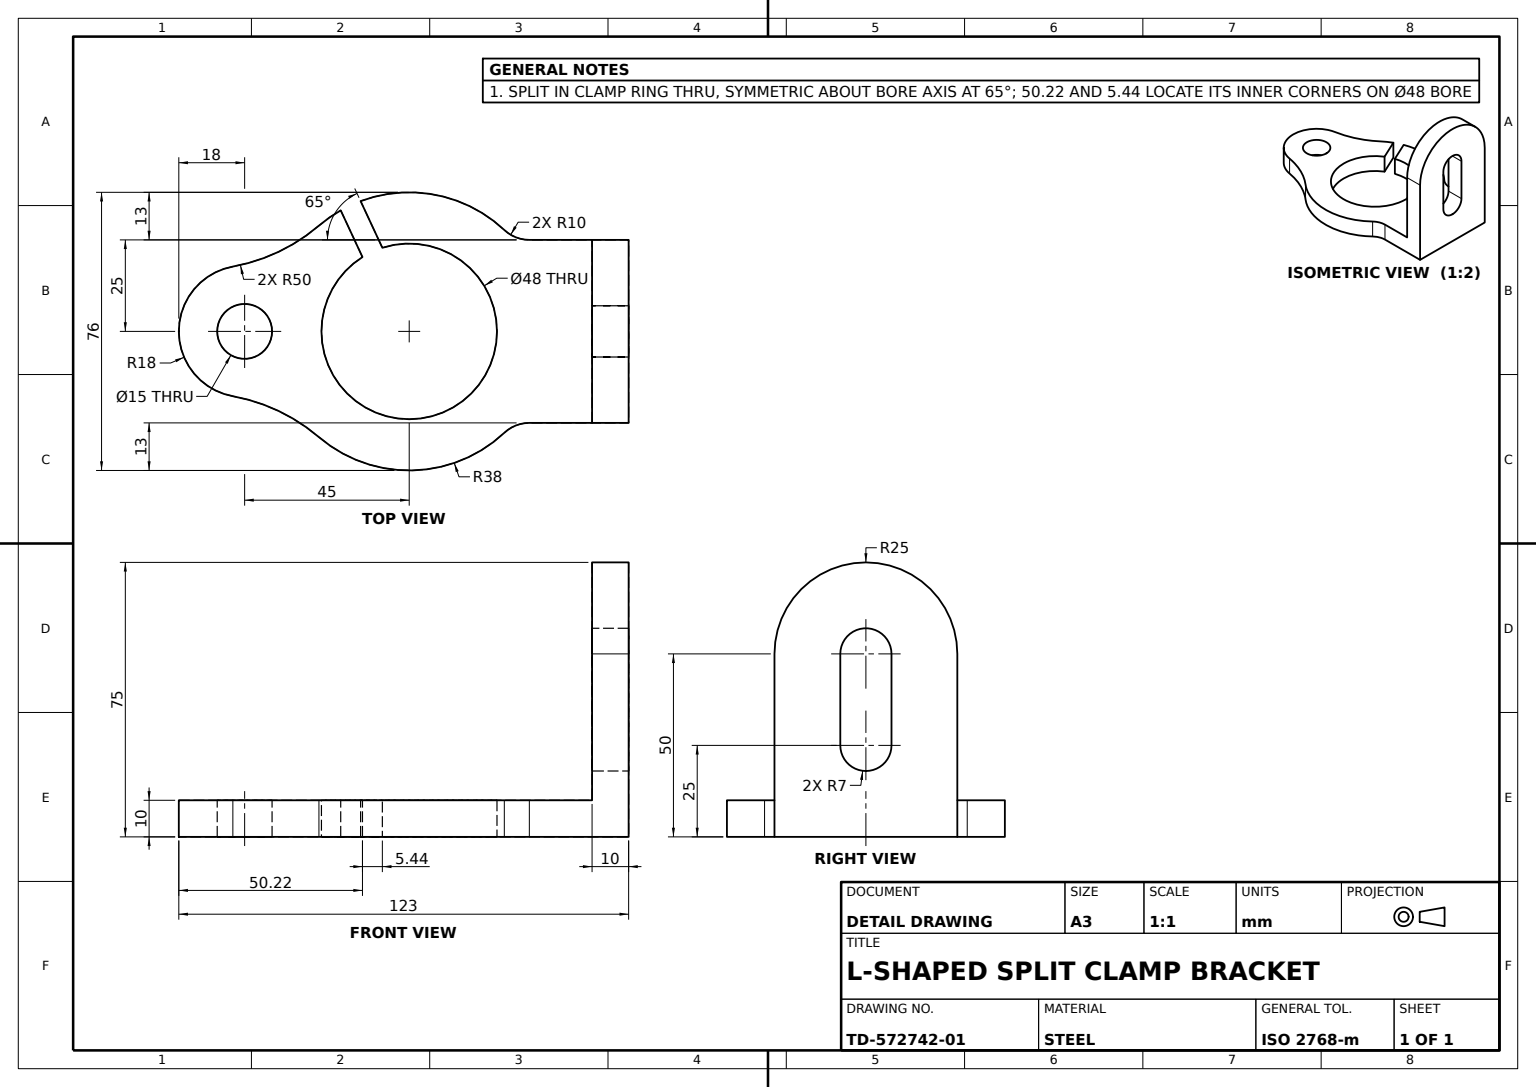
from build123d import *

# Parameters (mm, degrees)
L_ANGLE_PROFILE_SKETCH_W       = 150
L_ANGLE_PROFILE_SKETCH_H       = 10
L_ANGLE_PROFILE_SKETCH_W_2     = 10
L_ANGLE_PROFILE_SKETCH_H_2     = 100
L_ANGLE_BASE_DEPTH             = 43
UPRIGHT_TAB_AND_SLOT_CUT_DEPTH = 116
CLAMP_ARM_PROFILE_SKETCH_R     = 7.5
CLAMP_ARM_PROFILE_CUT_DEPTH    = 116


with BuildPart() as part:
    # L-Angle Profile Sketch → L-Angle Base (new, symmetric)
    with BuildSketch(Plane.XY):
        with Locations((-75, 5)):
            Rectangle(L_ANGLE_PROFILE_SKETCH_W, L_ANGLE_PROFILE_SKETCH_H)
        with Locations((5, 50)):
            Rectangle(L_ANGLE_PROFILE_SKETCH_W_2, L_ANGLE_PROFILE_SKETCH_H_2)
    extrude(amount=L_ANGLE_BASE_DEPTH, both=True)

    # Upright Tab and Slot Sketch → Upright Tab and Slot Cut (cut)
    with BuildSketch(Plane.ZY):
        with BuildLine():
            Line((7, 50), (7, 25))
            ThreePointArc((7, 25), (0, 18), (-7, 25))
            Line((-7, 25), (-7, 50))
            ThreePointArc((-7, 50), (0, 57), (7, 50))
        make_face()
        with BuildLine():
            Line((-25, 50), (-25, 10))
            Line((-25, 10), (-59.506944139, 10))
            Line((-59.506944139, 10), (-59.506944139, 107.254315339))
            Line((-59.506944139, 107.254315339), (43, 107.254315339))
            Line((43, 107.254315339), (43, 10))
            Line((43, 10), (25, 10))
            Line((25, 10), (25, 50))
            ThreePointArc((25, 50), (0, 75), (-25, 50))
        make_face()
    extrude(amount=-UPRIGHT_TAB_AND_SLOT_CUT_DEPTH, mode=Mode.SUBTRACT)

    # Clamp Arm Profile Sketch → Clamp Arm Profile Cut (cut)
    with BuildSketch(Plane(origin=(0, 10, 0), x_dir=(1, 0, 0), z_dir=(0, 1, 0))):
        with Locations(Location((-95, 0, 0), (0, 0, 180))):
            Circle(CLAMP_ARM_PROFILE_SKETCH_R)
        with BuildLine():
            Line((10, -25), (10, -43))
            Line((10, -43), (-150, -43))
            Line((-150, -43), (-150, 43))
            Line((-150, 43), (10, 43))
            Line((10, 43), (10, 25))
            Line((10, 25), (-17.151864589, 25))
            ThreePointArc((-17.151864589, 25), (-20.83176495, 25.701702665), (-23.995226133, 27.708333333))
            ThreePointArc((-23.995226133, 27.708333333), (-42.517796957, 37.256095308), (-63.29044546, 35.600057015))
            Line((-63.29044546, 35.600057015), (-57.34436202, 22.848639927))
            ThreePointArc((-57.34436202, 22.848639927), (-39.857161718, -21.751386889), (-62.782208742, 20.312930357))
            Line((-62.782208742, 20.312930357), (-68.728292182, 33.064347445))
            ThreePointArc((-68.728292182, 33.064347445), (-71.807070885, 31.119955968), (-74.685606061, 28.889805354))
            ThreePointArc((-74.685606061, 28.889805354), (-85.712027428, 21.739686255), (-98.220588235, 17.709540124))
            ThreePointArc((-98.220588235, 17.709540124), (-113, 0), (-98.220588235, -17.709540124))
            ThreePointArc((-98.220588235, -17.709540124), (-85.712027428, -21.739686255), (-74.685606061, -28.889805354))
            ThreePointArc((-74.685606061, -28.889805354), (-49.114550984, -37.989682547), (-23.995226133, -27.708333333))
            ThreePointArc((-23.995226133, -27.708333333), (-20.83176495, -25.701702665), (-17.151864589, -25))
            Line((-17.151864589, -25), (10, -25))
        make_face()
    extrude(amount=-CLAMP_ARM_PROFILE_CUT_DEPTH, mode=Mode.SUBTRACT)


solid = part.part
